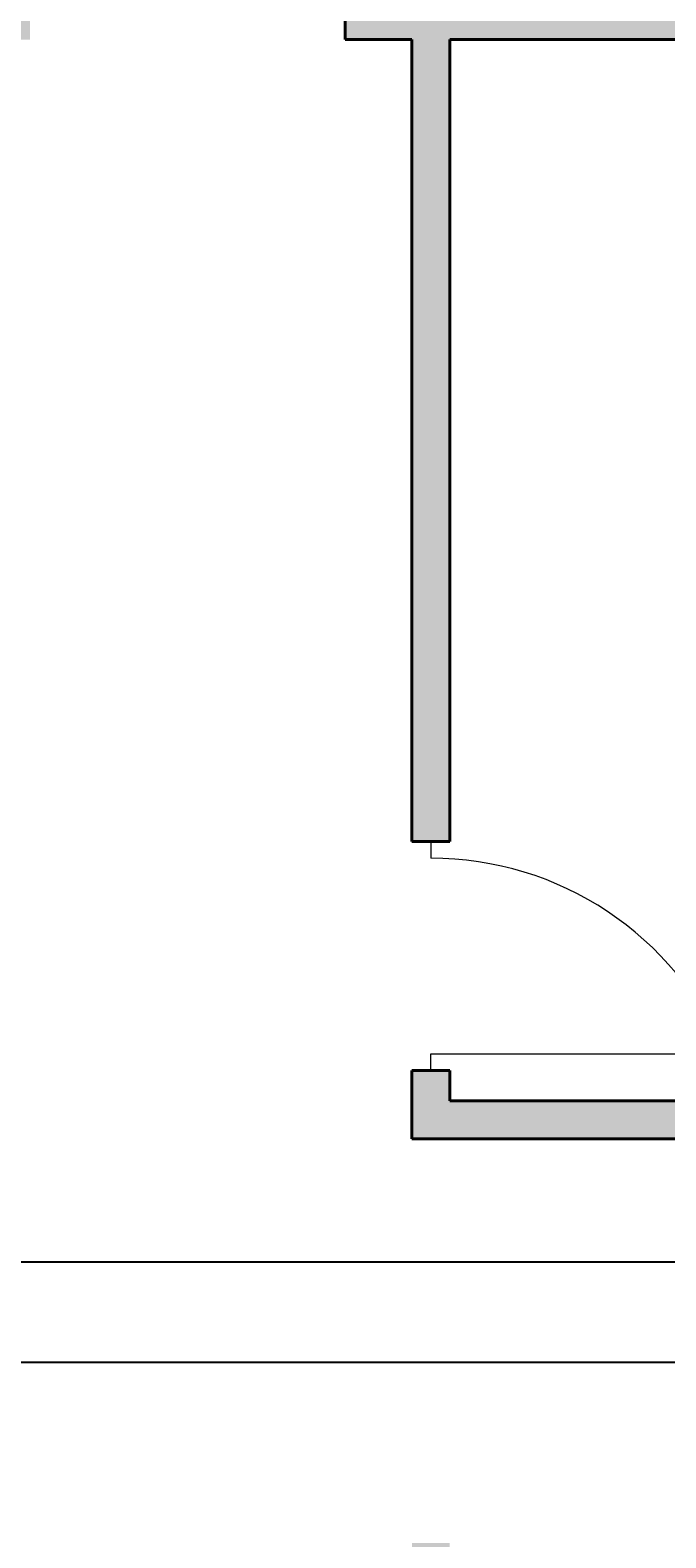
# Model space of a CAD drawing. Units: inches. Extents: x 1441 to 2460, y 1648 to 2683.
# Tile 13 of 35: x 1711 to 1786, y 1975 to 2154. Entities that reach past the tile are written whole.
import ezdxf

# ---------------------------------------------------------------- set-up
doc = ezdxf.new("R2010")
doc.units = ezdxf.units.IN
for name, color, linetype, lineweight in [('A-ANNO-DIMS', 2, 'Continuous', 18), ('A-DOOR', 3, 'Continuous', 20), ('A-WALL', 7, 'Continuous', 40)]:
    doc.layers.add(name, color=color, linetype=linetype, lineweight=lineweight)
doc.layers.add('A-WALL-PATT', color=251, linetype='Continuous', lineweight=13, true_color=0x636466)
doc.styles.get("Standard").update_dxf_attribs({"font": 'arial.ttf'})
doc.dimstyles.get("Standard").update_dxf_attribs({"dimtxt": 0.18, "dimasz": 0.18, "dimexe": 0.18, "dimexo": 0.0625, "dimgap": 0.09, "dimtad": 0, "dimtih": 1, "dimtoh": 1, "dimdec": 4, "dimzin": 0, "dimdsep": 46, "dimtxsty": 'Standard', "dimcen": 0.09, "dimadec": 0, "dimazin": 0, "dimtfac": 1, "dimtdec": 4, "dimtofl": 0, "dimtmove": 0, "dimatfit": 3, "dimfxl": 1, "dimtolj": 1, "dimtzin": 0, "dimarcsym": 0})

# ---------------------------------------------------------------- blocks, each defined once
blk = doc.blocks.new('DOOR-BED2-30')
for p, q in [((0, 27.22), (0, 25.22)), ((0, 0), (0, 2)), ((0, 2), (4.91, 2)), ((4.91, 2), (34.91, 2))]:
    blk.add_line(p, q)
blk.add_arc((0, -12.65), 37.87, 22.7676, 90)
blk = doc.blocks.new('*D67')
at = {"layer": 'A-ANNO-DIMS', "color": 0, "lineweight": -2, "transparency": 16777216}
for p, q in [((1889.45, 2298.7), (1916.22, 2298.7)), ((1916.04, 2298.52), (1916.04, 2055.94)), ((1916.04, 1813), (1916.04, 2055.57)), ((1758.22, 1812.82), (1916.22, 1812.82))]:
    blk.add_line(p, q, dxfattribs=at)
at = {"layer": 'A-ANNO-DIMS', "color": 0, "transparency": 16777216}
for points in [[(1916.01, 2298.52), (1916.07, 2298.52), (1916.04, 2298.7)], [(1916.01, 1813), (1916.07, 1813), (1916.04, 1812.82)]]:
    blk.add_solid(points, dxfattribs=at)
at = {"layer": 'Defpoints', "color": 0, "transparency": 16777216}
for p in [(1889.39, 2298.7), (1916.04, 2298.7), (1758.16, 1812.82)]:
    blk.add_point(p, dxfattribs=at)
at = {"layer": 'A-ANNO-DIMS', "color": 0, "transparency": 16777216, "insert": (1916.04, 2055.76), "char_height": 0.18, "attachment_point": 5}
blk.add_mtext('\\A1;485.9', dxfattribs=at)
blk = doc.blocks.new('*D125')
at = {"layer": 'A-ANNO-DIMS', "color": 0, "lineweight": -2, "transparency": 16777216}
for p, q in [((1616.11, 2008.09), (1916.22, 2008.09)), ((1916.04, 2007.91), (1916.04, 2002.31)), ((1916.04, 1996.35), (1916.04, 2001.95)), ((1616.11, 1996.17), (1916.22, 1996.17))]:
    blk.add_line(p, q, dxfattribs=at)
at = {"layer": 'A-ANNO-DIMS', "color": 0, "transparency": 16777216}
for points in [[(1916.01, 2007.91), (1916.07, 2007.91), (1916.04, 2008.09)], [(1916.01, 1996.35), (1916.07, 1996.35), (1916.04, 1996.17)]]:
    blk.add_solid(points, dxfattribs=at)
at = {"layer": 'Defpoints', "color": 0, "transparency": 16777216}
for p in [(1616.05, 2008.09), (1916.04, 2008.09), (1616.05, 1996.17)]:
    blk.add_point(p, dxfattribs=at)
at = {"layer": 'A-ANNO-DIMS', "color": 0, "transparency": 16777216, "insert": (1916.04, 2002.13), "char_height": 0.18, "attachment_point": 5}
blk.add_mtext('\\A1;11.922', dxfattribs=at)

msp = doc.modelspace()

# ---------------------------------------------------------------- hatches: boundary and pattern name
at = {"layer": 'A-WALL-PATT'}
h = msp.add_hatch(color=256, dxfattribs=at)
h.dxf.hatch_style = 1
h.paths.add_polyline_path([(1627.5085, 2298.6952), (1568.8859, 2298.6952), (1568.8859, 2246.9605), (1577.8859, 2246.9605), (1577.8859, 2289.6952), (1627.5085, 2289.6952), (1627.5085, 2294.1952)])
h.paths.add_polyline_path([(1675.5777, 2298.6952), (1651.5085, 2298.6952), (1651.5085, 2289.6952), (1675.5777, 2289.6952), (1675.5777, 2294.1952)])
h.paths.add_polyline_path([(1667.3859, 2289.6952), (1662.8859, 2289.6952), (1662.8859, 2233.0622), (1667.3859, 2233.0622)])
h.paths.add_polyline_path([(1715.8721, 2294.3362), (1715.8721, 2295.2788), (1715.8721, 2298.6952), (1699.5777, 2298.6952), (1699.5777, 2289.6952), (1715.8721, 2289.6952)])
h.paths.add_polyline_path([(1707.8859, 2289.6952), (1703.3859, 2289.6952), (1703.3859, 2199.6952), (1707.8859, 2199.6952)])
h.paths.add_polyline_path([(1760.3859, 2204.637), (1755.8859, 2204.637), (1755.8859, 2199.6952), (1667.3859, 2199.6952), (1667.3859, 2204.637), (1662.8859, 2204.637), (1662.8859, 2195.1952), (1760.3859, 2195.1952)])
h.paths.add_polyline_path([(1760.3859, 2289.6952), (1755.8859, 2289.6952), (1755.8859, 2233.0622), (1760.3859, 2233.0622)])
h.paths.add_polyline_path([(1889.3859, 2298.6952), (1739.8721, 2298.6952), (1739.8721, 2289.6952), (1880.3859, 2289.6952), (1880.3859, 2250.8051), (1889.3859, 2250.8051)])
h.paths.add_polyline_path([(1889.3859, 2202.8051), (1880.3859, 2202.8051), (1880.3859, 2157.6952), (1747.948, 2157.6952), (1747.948, 2153.1952), (1755.8859, 2153.1952), (1755.8859, 2058.005), (1760.3859, 2058.005), (1760.3859, 2153.1952), (1880.3859, 2153.1952), (1880.3859, 2124.108), (1889.3859, 2124.108)])
h.paths.add_polyline_path([(1889.3859, 1984.8305), (1880.3859, 1984.8305), (1880.3859, 1834.1952), (1889.3859, 1834.1952)])
h.paths.add_polyline_path([(1889.3859, 2076.108), (1880.3859, 2076.108), (1880.3859, 2008.8305), (1889.3859, 2008.8305)])
h.paths.add_polyline_path([(1880.3859, 2027.1952), (1800.8859, 2027.1952), (1800.8859, 2000.9452), (1805.3859, 2000.9452), (1805.3859, 2022.6952), (1880.3859, 2022.6952)])
h.paths.add_polyline_path([(1800.8859, 2027.1952), (1760.3859, 2027.1952), (1760.3859, 2030.7912), (1755.8859, 2030.7912), (1755.8859, 2022.6952), (1800.8859, 2022.6952)])
h.paths.add_polyline_path([(1880.3859, 1974.6952), (1805.3859, 1974.6952), (1805.3859, 1978.7973), (1800.8859, 1978.7973), (1800.8859, 1974.6952), (1794.8823, 1974.6952), (1794.8823, 1970.1952), (1800.8859, 1970.1952), (1805.3859, 1970.1952), (1880.3859, 1970.1952)])
h.paths.add_polyline_path([(1760.3859, 1974.6952), (1755.8859, 1974.6952), (1755.8859, 1925.6952), (1751.8616, 1925.6952), (1751.8616, 1921.1952), (1760.3859, 1921.1952)])
h.paths.add_polyline_path([(1760.3859, 1921.1952), (1755.8859, 1921.1952), (1755.8859, 1843.1952), (1760.3859, 1843.1952)])
h.paths.add_polyline_path([(1799.1136, 1838.6952), (1799.1136, 1843.1952), (1760.3859, 1843.1952), (1751.8944, 1843.1952), (1751.8944, 1834.1952), (1758.1615, 1834.1952), (1799.1136, 1834.1952)])
h.paths.add_polyline_path([(1880.3859, 1843.1952), (1859.1136, 1843.1952), (1859.1136, 1834.1952), (1880.3859, 1834.1952)])
h.paths.add_polyline_path([(1577.8859, 1857.7914), (1568.8859, 1857.7914), (1568.8859, 1834.1952), (1695.0034, 1834.1952), (1695.0034, 1838.6952), (1695.0034, 1843.1952), (1577.8859, 1843.1952)])
h.paths.add_polyline_path([(1577.8859, 1959.2399), (1573.3859, 1959.2399), (1568.8859, 1959.2399), (1568.8859, 1905.7914), (1577.8859, 1905.7914), (1577.8859, 1921.1952), (1703.3859, 1921.1952), (1707.8859, 1921.1952), (1715.1501, 1921.1952), (1715.1501, 1925.6952), (1707.8859, 1925.6952), (1703.3859, 1925.6952), (1577.8859, 1925.6952)])
h.paths.add_polyline_path([(1577.8859, 2106.6907), (1568.8859, 2106.6907), (1568.8859, 2019.2399), (1577.8859, 2019.2399)])
h.paths.add_polyline_path([(1707.8859, 2051.6952), (1703.3859, 2051.6952), (1703.3859, 2048.6952), (1703.3859, 1925.6952), (1707.8859, 1925.6952)])
h.paths.add_polyline_path([(1703.3859, 2051.6952), (1676.3859, 2051.6952), (1676.3859, 2048.6952), (1703.3859, 2048.6952)])
h.paths.add_polyline_path([(1703.3859, 2102.6952), (1676.3859, 2102.6952), (1676.3859, 2099.6952), (1685.3859, 2099.6952), (1703.3859, 2099.6952)])
h.paths.add_polyline_path([(1707.8859, 2153.1952), (1710.5611, 2153.1952), (1710.5611, 2157.6952), (1707.8859, 2157.6952), (1707.8859, 2195.1952), (1703.3859, 2195.1952), (1703.3859, 2099.6952), (1707.8859, 2099.6952)])
h.paths.add_polyline_path([(1577.8859, 2198.9605), (1568.8859, 2198.9605), (1568.8859, 2166.6907), (1577.8859, 2166.6907)])

# ---------------------------------------------------------------- linework, layer by layer
at = {"layer": 'A-WALL'}
for p, q in [((1747.948, 2157.6952), (1747.948, 2153.1952)), ((1747.948, 2153.1952), (1755.8859, 2153.1952)), ((1755.8859, 2153.1952), (1755.8859, 2058.005)), ((1760.3859, 2153.1952), (1760.3859, 2058.005)), ((1760.3859, 2153.1952), (1880.3859, 2153.1952)), ((1755.8859, 2058.005), (1760.3859, 2058.005)), ((1755.8859, 2030.7912), (1760.3859, 2030.7912)), ((1755.8859, 2030.7912), (1755.8859, 2022.6952)), ((1760.3859, 2030.7912), (1760.3859, 2027.1952)), ((1760.3859, 2027.1952), (1880.3859, 2027.1952)), ((1755.8859, 2022.6952), (1800.8859, 2022.6952))]:
    msp.add_line(p, q, dxfattribs=at)

# ---------------------------------------------------------------- block references
at = {"layer": 'A-DOOR'}
msp.add_blockref('DOOR-BED2-30', (1758.14, 2030.79), dxfattribs=at)

# ---------------------------------------------------------------- dimensions: what is measured, and where the dimension line sits
at = {"layer": 'A-ANNO-DIMS'}
for base, p1, p2, override, picture, middle in [((1916.0359, 2298.6952), (1758.1615, 1812.8171), (1889.3859, 2298.6952), {"dimdec": 1, "dimlfac": 1, "dimrnd": 0, "dimzin": 0, "dimdsep": 46, "dimlunit": 2}, '*D67', (1916.0359, 2055.7561)), ((1916.0359, 2008.0936), (1616.0509, 1996.172), (1616.0509, 2008.0936), {"dimdec": 3, "dimlfac": 1, "dimrnd": 0, "dimzin": 0, "dimdsep": 46, "dimlunit": 2}, '*D125', (1916.0359, 2002.1328))]:
    dim = msp.add_linear_dim(base=base, p1=p1, p2=p2, angle=90, dimstyle='Standard', override=override, dxfattribs=at)
    dim.commit()
    dim.dimension.update_dxf_attribs({"geometry": picture, "text_midpoint": middle})

doc.saveas('drawing.dxf')
